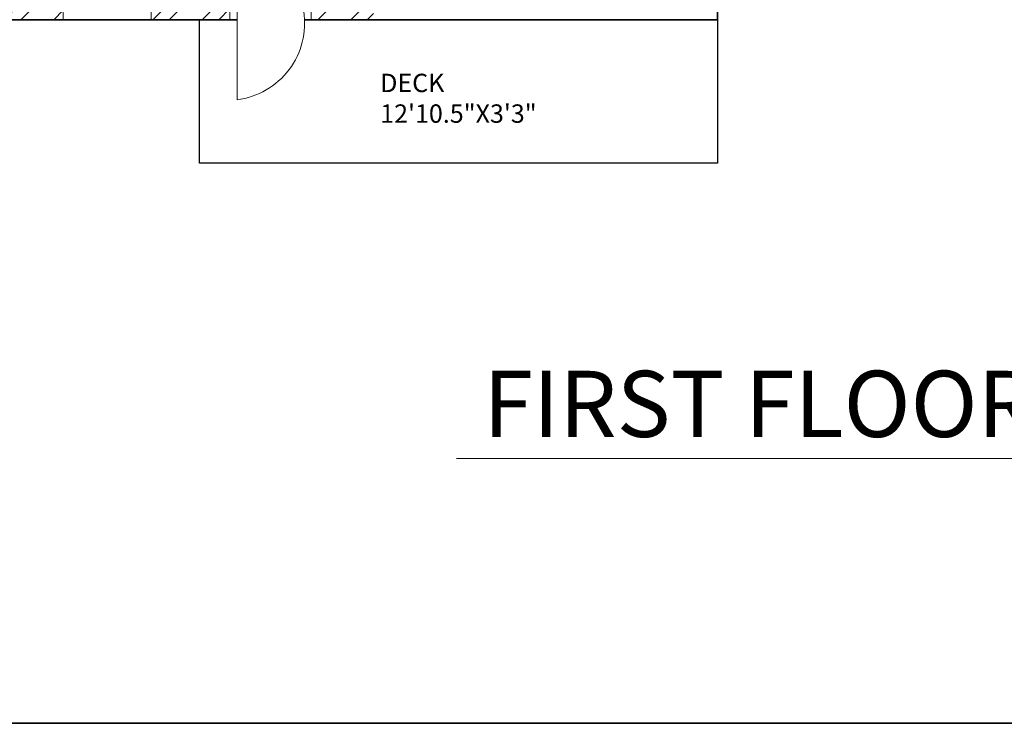
# Model space of a CAD drawing. Units: inches. Extents: x 2120 to 4013, y 1390 to 3019.
# Tile 9 of 59: x 2448 to 2716, y 1390 to 1582. Entities that reach past the tile are written whole.
import ezdxf

# ---------------------------------------------------------------- set-up
doc = ezdxf.new("R2010")
doc.units = ezdxf.units.IN
for name, color, linetype, lineweight in [('A-ANNO-TEXT', 7, 'Continuous', 18), ('A-ANNO-TTLB', 7, 'Continuous', 35), ('A-AREA-IDEN', 7, 'Continuous', 18), ('A-DOOR', 3, 'Continuous', 18), ('A-FLOR-DECK', 7, 'Continuous', 25), ('A-GLAZ', 4, 'Continuous', 18), ('A-WALL', 7, 'Continuous', 35), ('A-WALL-PATT', 252, 'Continuous', 13)]:
    doc.layers.add(name, color=color, linetype=linetype, lineweight=lineweight)
doc.styles.get("Standard").update_dxf_attribs({"font": 'arial.ttf'})

# ---------------------------------------------------------------- blocks, each defined once
blk = doc.blocks.new('DOOR-SWING-24IN-91p57DEG')
for p, q in [((0, 26.25), (0, 21.75)), ((22.12, 21.75), (22.12, 26.25)), ((22.12, 26.25), (22.12, 24)), ((0, 21.75), (0, 24)), ((0, 24), (2, 24)), ((2, 24), (2, 0)), ((22.12, 24), (20.12, 24))]:
    blk.add_line(p, q)
blk.add_arc((-0.62, 20.81), 20.98, 277.1643, 8.7385)
blk = doc.blocks.new('WIN-PLAN-24IN-03')
for p, q in [((9, 24), (0, 24)), ((0, 24), (4.5, 24)), ((4.5, 24), (4.5, 0)), ((9, 0), (0, 0)), ((4.5, 0), (9, 0))]:
    blk.add_line(p, q)

msp = doc.modelspace()

# ---------------------------------------------------------------- hatches: boundary and pattern name
at = {"layer": 'A-WALL-PATT'}
h = msp.add_hatch(dxfattribs=at)
h.set_pattern_fill('ANSI32', color=256)
h.paths.add_polyline_path([(2271.7331, 2343.531), (2283.3788, 2343.531), (2283.3788, 2348.031), (2283.3788, 2352.5306), (2262.7331, 2352.5306), (2262.7331, 2182.638), (2267.2331, 2182.638), (2271.7331, 2182.638), (2271.7331, 2219.031), (2391.7331, 2219.031), (2391.7331, 2214.189), (2393.9831, 2214.189), (2396.2331, 2214.189), (2396.2331, 2219.031), (2420.2331, 2219.031), (2420.2331, 2225.7535), (2417.2197, 2225.7535), (2415.7331, 2225.7535), (2415.7331, 2223.5306), (2271.7331, 2223.5306)])
h.paths.add_polyline_path([(2380.0942, 2352.5306), (2343.3788, 2352.5306), (2343.3788, 2343.531), (2363.2331, 2343.531), (2363.2331, 2288.8489), (2365.4831, 2288.8489), (2367.7331, 2288.8489), (2367.7331, 2343.531), (2380.0942, 2343.531)], flags=17)
h.paths.add_polyline_path([(2432.4339, 2352.5306), (2404.0943, 2352.5306), (2404.0943, 2343.531), (2415.7331, 2343.531), (2415.7331, 2264.0306), (2367.7331, 2264.0306), (2367.7331, 2266.4872), (2363.2331, 2266.4872), (2363.2331, 2259.531), (2367.7331, 2259.531), (2415.7331, 2259.531), (2415.7331, 2255.0658), (2420.2331, 2255.0658), (2420.2331, 2259.531), (2424.5717, 2259.531), (2424.5717, 2261.781), (2424.5717, 2264.0306), (2420.2331, 2264.0306), (2420.2331, 2343.531), (2432.4339, 2343.531)])
h.paths.add_polyline_path([(2508.9115, 2352.5306), (2456.4339, 2352.5306), (2456.4339, 2343.531), (2468.2331, 2343.531), (2468.2331, 2264.0306), (2448.0487, 2264.0306), (2448.0487, 2259.531), (2468.2331, 2259.531), (2468.2331, 2255.5496), (2472.7331, 2255.5496), (2472.7331, 2343.531), (2508.9115, 2343.531)])
h.paths.add_polyline_path([(2637.7331, 2352.5306), (2544.9116, 2352.5306), (2544.9116, 2343.531), (2589.7331, 2343.531), (2633.2331, 2343.531), (2637.7331, 2343.531)])
h.paths.add_polyline_path([(2594.2331, 2343.5306), (2589.7331, 2343.5306), (2589.7331, 2259.5306), (2589.7331, 2252.4915), (2591.9831, 2252.4915), (2594.2331, 2252.4915)])
h.paths.add_polyline_path([(2637.7331, 2223.5306), (2594.2331, 2223.5306), (2594.2331, 2230.1988), (2591.9831, 2230.1988), (2589.7331, 2230.1988), (2589.7331, 2223.5306), (2472.7331, 2223.5306), (2468.2331, 2223.5306), (2468.2331, 2219.031), (2628.7331, 2219.031), (2628.7331, 2138.031), (2637.7331, 2138.031)])
h.paths.add_polyline_path([(3822.6535, 2458.4402), (3874.9468, 2458.4402), (3874.9468, 2476.9866), (3822.6535, 2476.9866)], flags=9)
h.paths.add_polyline_path([(3834.6921, 2781.8174), (3935.9206, 2781.8174), (3935.9206, 2800.3638), (3834.6921, 2800.3638)], flags=9)
h.paths.add_polyline_path([(3832.2843, 2837.9683), (3884.5776, 2837.9683), (3884.5776, 2856.5146), (3832.2843, 2856.5146)], flags=9)
h.paths.add_polyline_path([(3830.9388, 2861.4782), (3956.8958, 2861.4782), (3956.8958, 2880.0245), (3830.9388, 2880.0245)], flags=9)
h.paths.add_polyline_path([(3870.6966, 2352.5752), (3887.9272, 2352.5752), (3887.9272, 2377.3037), (3870.6966, 2377.3037)], flags=9)
h.paths.add_polyline_path([(3289.2701, 2413.161), (3435.2223, 2413.161), (3435.2223, 2450.2538), (3289.2701, 2450.2538)], flags=9)
h.paths.add_polyline_path([(2487.6944, 2414.3601), (2637.8335, 2414.3601), (2637.8335, 2451.4528), (2487.6944, 2451.4528)], flags=9)
h.paths.add_polyline_path([(2567.3724, 1457.9199), (2815.296, 1457.9199), (2815.296, 1495.0127), (2567.3724, 1495.0127)], flags=9)
h.paths.add_polyline_path([(2655.3825, 2093.2363), (2685.9555, 2093.2363), (2685.9555, 2111.8937), (2655.3825, 2111.8937)], flags=9)
h.paths.add_polyline_path([(2543.9218, 1550.6671), (2587.8406, 1550.6671), (2587.8406, 1569.3244), (2543.9218, 1569.3244)], flags=9)
h.paths.add_polyline_path([(2905.1384, 1543.8113), (2949.0572, 1543.8113), (2949.0572, 1562.4686), (2905.1384, 1562.4686)], flags=9)
h.paths.add_polyline_path([(2736.4118, 1702.4736), (2784.2153, 1702.4736), (2784.2153, 1721.1309), (2736.4118, 1721.1309)], flags=9)
h.paths.add_polyline_path([(2912.8666, 1710.4168), (2951.707, 1710.4168), (2951.707, 1729.0741), (2912.8666, 1729.0741)], flags=9)
h.paths.add_polyline_path([(2923.5785, 1763.5038), (2959.7279, 1763.5038), (2959.7279, 1782.1611), (2923.5785, 1782.1611)], flags=9)
h.paths.add_polyline_path([(2925.2114, 1809.6137), (2967.1861, 1809.6137), (2967.1861, 1828.271), (2925.2114, 1828.271)], flags=9)
h.paths.add_polyline_path([(2996.2711, 1878.9003), (2996.2711, 1913.109), (2977.6138, 1913.109), (2977.6138, 1878.9003)], flags=9)
h.paths.add_polyline_path([(2883.0859, 1895.7192), (2927.1855, 1895.7192), (2927.1855, 1914.3766), (2883.0859, 1914.3766)], flags=9)
h.paths.add_polyline_path([(2787.3924, 1810.8013), (2841.0213, 1810.8013), (2841.0213, 1829.4587), (2787.3924, 1829.4587)], flags=9)
h.paths.add_polyline_path([(2775.6399, 2101.7395), (2829.2689, 2101.7395), (2829.2689, 2120.3968), (2775.6399, 2120.3968)], flags=9)
h.paths.add_polyline_path([(2913.0263, 2075.817), (2951.8667, 2075.817), (2951.8667, 2094.4744), (2913.0263, 2094.4744)], flags=9)
h.paths.add_polyline_path([(2929.966, 2133.3669), (2966.1154, 2133.3669), (2966.1154, 2152.0243), (2929.966, 2152.0243)], flags=9)
h.paths.add_polyline_path([(2932.7502, 2182.6088), (2968.8996, 2182.6088), (2968.8996, 2201.2662), (2932.7502, 2201.2662)], flags=9)
h.paths.add_polyline_path([(2996.0681, 2266.3173), (2996.0681, 2300.5261), (2977.4108, 2300.5261), (2977.4108, 2266.3173)], flags=9)
h.paths.add_polyline_path([(2885.1039, 2279.2186), (2929.2035, 2279.2186), (2929.2035, 2297.8759), (2885.1039, 2297.8759)], flags=9)
h.paths.add_polyline_path([(2735.7042, 2218.3197), (2783.5078, 2218.3197), (2783.5078, 2236.9771), (2735.7042, 2236.9771)], flags=9)
h.paths.add_polyline_path([(2635.6049, 2044.0085), (2648.9678, 2044.0085), (2648.9678, 2054.312), (2635.6049, 2054.312)], flags=9)
h.paths.add_polyline_path([(2714.0148, 1923.0473), (2727.3777, 1923.0473), (2727.3777, 1933.3508), (2714.0148, 1933.3508)], flags=9)
h.paths.add_polyline_path([(2709.0345, 1988.1628), (2722.3974, 1988.1628), (2722.3974, 1998.4663), (2709.0345, 1998.4663)], flags=9)
h.paths.add_polyline_path([(2592.8935, 1962.1763), (2606.2564, 1962.1763), (2606.2564, 1972.4799), (2592.8935, 1972.4799)], flags=9)
h.paths.add_polyline_path([(2618.3996, 1985.9724), (2644.1942, 1985.9724), (2644.1942, 1996.2759), (2618.3996, 1996.2759)], flags=9)
h.paths.add_polyline_path([(2601.279, 1920.5869), (2614.6419, 1920.5869), (2614.6419, 1930.8904), (2601.279, 1930.8904)], flags=9)
h.paths.add_polyline_path([(2692.3278, 1932.7645), (2704.5311, 1932.7645), (2704.5311, 1943.0681), (2692.3278, 1943.0681)], flags=9)
h.paths.add_polyline_path([(2311.122, 1672.7318), (2355.0408, 1672.7318), (2355.0408, 1691.3892), (2311.122, 1691.3892)], flags=9)
h.paths.add_polyline_path([(2456.2551, 1632.3198), (2492.4796, 1632.3198), (2492.4796, 1650.9772), (2456.2551, 1650.9772)], flags=9)
h.paths.add_polyline_path([(2401.0766, 1631.4793), (2437.301, 1631.4793), (2437.301, 1650.1367), (2401.0766, 1650.1367)], flags=9)
h.paths.add_polyline_path([(2546.7054, 1700.9235), (2594.509, 1700.9235), (2594.509, 1719.5809), (2546.7054, 1719.5809)], flags=9)
h.paths.add_polyline_path([(2445.4866, 1766.9937), (2497.5261, 1766.9937), (2497.5261, 1785.651), (2445.4866, 1785.651)], flags=9)
h.paths.add_polyline_path([(2287.9992, 1739.7675), (2326.8396, 1739.7675), (2326.8396, 1758.4248), (2287.9992, 1758.4248)], flags=9)
h.paths.add_polyline_path([(2458.5279, 1924.7607), (2510.5675, 1924.7607), (2510.5675, 1943.4181), (2458.5279, 1943.4181)], flags=9)
h.paths.add_polyline_path([(2309.2811, 1902.7642), (2345.4305, 1902.7642), (2345.4305, 1921.4215), (2309.2811, 1921.4215)], flags=9)
h.paths.add_polyline_path([(2490.7554, 2018.9392), (2530.7896, 2018.9392), (2530.7896, 2037.5965), (2490.7554, 2037.5965)], flags=9)
h.paths.add_polyline_path([(2402.143, 2024.7393), (2438.5414, 2024.7393), (2438.5414, 2043.3966), (2402.143, 2043.3966)], flags=9)
h.paths.add_polyline_path([(2287.856, 1931.7926), (2326.6964, 1931.7926), (2326.6964, 1950.4499), (2287.856, 1950.4499)], flags=9)
h.paths.add_polyline_path([(2281.7979, 2193.5771), (2320.6383, 2193.5771), (2320.6383, 2212.2344), (2281.7979, 2212.2344)], flags=25)
h.paths.add_polyline_path([(2484.0754, 2093.892), (2536.115, 2093.892), (2536.115, 2112.5494), (2484.0754, 2112.5494)], flags=9)
h.paths.add_polyline_path([(2624.7948, 2281.8639), (2624.7948, 2311.4137), (2606.1375, 2311.4137), (2606.1375, 2281.8639)], flags=9)
h.paths.add_polyline_path([(2507.5036, 2290.3639), (2541.934, 2290.3639), (2541.934, 2309.0212), (2507.5036, 2309.0212)], flags=9)
h.paths.add_polyline_path([(2423.1076, 2285.2202), (2459.332, 2285.2202), (2459.332, 2303.8776), (2423.1076, 2303.8776)], flags=9)
h.paths.add_polyline_path([(2374.5467, 2289.6272), (2410.7711, 2289.6272), (2410.7711, 2308.2846), (2374.5467, 2308.2846)], flags=25)
h.paths.add_polyline_path([(2277.4907, 2227.5651), (2316.3311, 2227.5651), (2316.3311, 2246.2224), (2277.4907, 2246.2224)], flags=25)
h.paths.add_polyline_path([(2655.3825, 2093.2367), (2685.9555, 2093.2367), (2685.9555, 2111.894), (2655.3825, 2111.894)], flags=9)
h.paths.add_polyline_path([(2543.9217, 1550.6674), (2587.8406, 1550.6674), (2587.8406, 1569.3247), (2543.9217, 1569.3247)], flags=9)
h.paths.add_polyline_path([(2905.1384, 1543.8116), (2949.0572, 1543.8116), (2949.0572, 1562.4689), (2905.1384, 1562.4689)], flags=9)
h.paths.add_polyline_path([(2736.4118, 1702.4739), (2784.2153, 1702.4739), (2784.2153, 1721.1312), (2736.4118, 1721.1312)], flags=9)
h.paths.add_polyline_path([(2912.8666, 1710.4171), (2951.707, 1710.4171), (2951.707, 1729.0744), (2912.8666, 1729.0744)], flags=9)
h.paths.add_polyline_path([(2923.5785, 1763.5041), (2959.7279, 1763.5041), (2959.7279, 1782.1614), (2923.5785, 1782.1614)], flags=9)
h.paths.add_polyline_path([(2925.2114, 1809.614), (2967.1861, 1809.614), (2967.1861, 1828.2713), (2925.2114, 1828.2713)], flags=9)
h.paths.add_polyline_path([(2996.2711, 1878.9006), (2996.2711, 1913.1094), (2977.6137, 1913.1094), (2977.6137, 1878.9006)], flags=9)
h.paths.add_polyline_path([(2883.0859, 1895.7195), (2927.1855, 1895.7195), (2927.1855, 1914.3769), (2883.0859, 1914.3769)], flags=9)
h.paths.add_polyline_path([(2787.3924, 1810.8016), (2841.0213, 1810.8016), (2841.0213, 1829.459), (2787.3924, 1829.459)], flags=9)
h.paths.add_polyline_path([(2775.6399, 2101.7398), (2829.2688, 2101.7398), (2829.2688, 2120.3971), (2775.6399, 2120.3971)], flags=9)
h.paths.add_polyline_path([(2913.0263, 2075.8173), (2951.8667, 2075.8173), (2951.8667, 2094.4747), (2913.0263, 2094.4747)], flags=9)
h.paths.add_polyline_path([(2929.966, 2133.3672), (2966.1154, 2133.3672), (2966.1154, 2152.0246), (2929.966, 2152.0246)], flags=9)
h.paths.add_polyline_path([(2932.7502, 2182.6091), (2968.8996, 2182.6091), (2968.8996, 2201.2665), (2932.7502, 2201.2665)], flags=9)
h.paths.add_polyline_path([(2996.0681, 2266.3176), (2996.0681, 2300.5264), (2977.4108, 2300.5264), (2977.4108, 2266.3176)], flags=9)
h.paths.add_polyline_path([(2885.1039, 2279.2189), (2929.2035, 2279.2189), (2929.2035, 2297.8762), (2885.1039, 2297.8762)], flags=9)
h.paths.add_polyline_path([(2735.7042, 2218.32), (2783.5078, 2218.32), (2783.5078, 2236.9774), (2735.7042, 2236.9774)], flags=9)
h.paths.add_polyline_path([(2635.6048, 2044.0088), (2648.9677, 2044.0088), (2648.9677, 2054.3123), (2635.6048, 2054.3123)], flags=9)
h.paths.add_polyline_path([(2714.0148, 1923.0476), (2727.3777, 1923.0476), (2727.3777, 1933.3511), (2714.0148, 1933.3511)], flags=9)
h.paths.add_polyline_path([(2709.0345, 1988.1631), (2722.3974, 1988.1631), (2722.3974, 1998.4666), (2709.0345, 1998.4666)], flags=9)
h.paths.add_polyline_path([(2592.8935, 1962.1766), (2606.2564, 1962.1766), (2606.2564, 1972.4802), (2592.8935, 1972.4802)], flags=9)
h.paths.add_polyline_path([(2618.3995, 1985.9727), (2644.1942, 1985.9727), (2644.1942, 1996.2762), (2618.3995, 1996.2762)], flags=9)
h.paths.add_polyline_path([(2601.279, 1920.5872), (2614.6419, 1920.5872), (2614.6419, 1930.8908), (2601.279, 1930.8908)], flags=9)
h.paths.add_polyline_path([(2692.3278, 1932.7648), (2704.5311, 1932.7648), (2704.5311, 1943.0684), (2692.3278, 1943.0684)], flags=9)
h.paths.add_polyline_path([(2311.122, 1672.7321), (2355.0408, 1672.7321), (2355.0408, 1691.3895), (2311.122, 1691.3895)], flags=9)
h.paths.add_polyline_path([(2456.2551, 1632.3201), (2492.4795, 1632.3201), (2492.4795, 1650.9775), (2456.2551, 1650.9775)], flags=9)
h.paths.add_polyline_path([(2401.0766, 1631.4796), (2437.301, 1631.4796), (2437.301, 1650.137), (2401.0766, 1650.137)], flags=9)
h.paths.add_polyline_path([(2546.7054, 1700.9238), (2594.509, 1700.9238), (2594.509, 1719.5812), (2546.7054, 1719.5812)], flags=9)
h.paths.add_polyline_path([(2445.4866, 1766.994), (2497.5261, 1766.994), (2497.5261, 1785.6513), (2445.4866, 1785.6513)], flags=9)
h.paths.add_polyline_path([(2287.9992, 1739.7678), (2326.8396, 1739.7678), (2326.8396, 1758.4251), (2287.9992, 1758.4251)], flags=9)
h.paths.add_polyline_path([(2458.5279, 1924.7611), (2510.5675, 1924.7611), (2510.5675, 1943.4184), (2458.5279, 1943.4184)], flags=9)
h.paths.add_polyline_path([(2309.2811, 1902.7645), (2345.4305, 1902.7645), (2345.4305, 1921.4218), (2309.2811, 1921.4218)], flags=9)
h.paths.add_polyline_path([(2490.7554, 2018.9395), (2530.7895, 2018.9395), (2530.7895, 2037.5968), (2490.7554, 2037.5968)], flags=9)
h.paths.add_polyline_path([(2402.143, 2024.7396), (2438.5413, 2024.7396), (2438.5413, 2043.3969), (2402.143, 2043.3969)], flags=9)
h.paths.add_polyline_path([(2287.856, 1931.7929), (2326.6964, 1931.7929), (2326.6964, 1950.4502), (2287.856, 1950.4502)], flags=9)
h.paths.add_polyline_path([(2281.7979, 2193.5774), (2320.6383, 2193.5774), (2320.6383, 2212.2347), (2281.7979, 2212.2347)], flags=25)
h.paths.add_polyline_path([(2484.0754, 2093.8924), (2536.115, 2093.8924), (2536.115, 2112.5497), (2484.0754, 2112.5497)], flags=9)
h.paths.add_polyline_path([(2624.7948, 2281.8642), (2624.7948, 2311.414), (2606.1374, 2311.414), (2606.1374, 2281.8642)], flags=9)
h.paths.add_polyline_path([(2507.5035, 2290.3642), (2541.934, 2290.3642), (2541.934, 2309.0215), (2507.5035, 2309.0215)], flags=9)
h.paths.add_polyline_path([(2423.1075, 2285.2205), (2459.332, 2285.2205), (2459.332, 2303.8779), (2423.1075, 2303.8779)], flags=9)
h.paths.add_polyline_path([(2374.5467, 2289.6275), (2410.7711, 2289.6275), (2410.7711, 2308.2849), (2374.5467, 2308.2849)], flags=25)
h.paths.add_polyline_path([(2277.4907, 2227.5654), (2316.3311, 2227.5654), (2316.3311, 2246.2227), (2277.4907, 2246.2227)], flags=25)
h = msp.add_hatch(dxfattribs=at)
h.set_pattern_fill('ANSI32', color=256)
h.paths.add_polyline_path([(2271.7331, 1980.389), (2262.7331, 1980.389), (2262.7331, 1912.8434), (2267.2331, 1912.8434), (2271.7331, 1912.8434), (2271.7331, 1922.531), (2351.2331, 1922.531), (2351.2331, 1901.4728), (2355.7331, 1901.4728), (2355.7331, 1922.531), (2357.9815, 1922.531), (2357.9815, 1926.5306), (2271.7331, 1926.5306)])
h.paths.add_polyline_path([(2589.2331, 1949.1622), (2584.7331, 1949.1622), (2580.2331, 1949.1622), (2580.2331, 1874.5306), (2355.7331, 1874.5306), (2355.7331, 1880.1922), (2351.2331, 1880.1922), (2351.2331, 1874.5306), (2271.7331, 1874.5306), (2271.7331, 1888.8431), (2262.7331, 1888.8431), (2262.7331, 1842.2909), (2267.2331, 1842.2909), (2271.7331, 1842.2909), (2271.7331, 1865.531), (2415.7331, 1865.531), (2415.7331, 1779.7286), (2420.2331, 1779.7286), (2420.2331, 1865.531), (2589.2331, 1865.531)])
h.paths.add_polyline_path([(2271.7331, 1782.2906), (2262.7331, 1782.2906), (2262.7331, 1711.4639), (2267.2331, 1711.4639), (2271.7331, 1711.4639), (2271.7331, 1738.031), (2420.2331, 1738.031), (2420.2331, 1742.531), (2420.2331, 1747.3376), (2417.9831, 1747.3376), (2415.7331, 1747.3376), (2415.7331, 1742.5306), (2271.7331, 1742.5306)])
h.paths.add_polyline_path([(2271.7331, 1627.031), (2362.3957, 1627.031), (2362.3957, 1629.281), (2362.3957, 1631.5306), (2271.7331, 1631.5306), (2271.7331, 1675.4636), (2262.7331, 1675.4636), (2262.7331, 1581.531), (2405.3032, 1581.531), (2405.3032, 1586.031), (2405.3032, 1590.5306), (2396.2331, 1590.5306), (2396.2331, 1691.4513), (2418.7206, 1691.4513), (2418.7206, 1695.951), (2396.2331, 1695.951), (2391.7331, 1695.951), (2391.7331, 1631.5306), (2386.7425, 1631.5306), (2386.7425, 1629.2806), (2386.7425, 1627.031), (2391.7331, 1627.031), (2391.7331, 1586.1709), (2271.7331, 1586.1709)])
h.paths.add_polyline_path([(2459.6703, 1590.5306), (2429.3032, 1590.5306), (2429.3032, 1581.531), (2459.6703, 1581.531), (2459.6703, 1586.031)])
h.paths.add_polyline_path([(2501.2331, 1590.531), (2501.2331, 1665.0195), (2498.9831, 1665.0195), (2496.7331, 1665.0195), (2496.7331, 1590.5306), (2483.8201, 1590.5306), (2483.8201, 1590.1579), (2483.6704, 1590.1579), (2483.6704, 1581.531), (2505.0196, 1581.531), (2505.0196, 1583.781), (2505.0196, 1586.0306), (2501.2331, 1586.0306)])
h.paths.add_polyline_path([(2544.1361, 1583.781), (2544.1361, 1586.0306), (2527.1368, 1586.0306), (2527.1368, 1583.7806), (2527.1368, 1581.531), (2544.1361, 1581.531)])
h.paths.add_polyline_path([(3822.6535, 2458.4402), (3874.9468, 2458.4402), (3874.9468, 2476.9866), (3822.6535, 2476.9866)], flags=9)
h.paths.add_polyline_path([(3834.6921, 2781.8174), (3935.9206, 2781.8174), (3935.9206, 2800.3638), (3834.6921, 2800.3638)], flags=9)
h.paths.add_polyline_path([(3832.2843, 2837.9683), (3884.5776, 2837.9683), (3884.5776, 2856.5146), (3832.2843, 2856.5146)], flags=9)
h.paths.add_polyline_path([(3830.9388, 2861.4782), (3956.8958, 2861.4782), (3956.8958, 2880.0245), (3830.9388, 2880.0245)], flags=9)
h.paths.add_polyline_path([(3870.6966, 2352.5752), (3887.9272, 2352.5752), (3887.9272, 2377.3037), (3870.6966, 2377.3037)], flags=9)
h.paths.add_polyline_path([(3289.2701, 2413.161), (3435.2223, 2413.161), (3435.2223, 2450.2538), (3289.2701, 2450.2538)], flags=9)
h.paths.add_polyline_path([(2487.6944, 2414.3601), (2637.8335, 2414.3601), (2637.8335, 2451.4528), (2487.6944, 2451.4528)], flags=9)
h.paths.add_polyline_path([(2567.3724, 1457.9199), (2815.296, 1457.9199), (2815.296, 1495.0127), (2567.3724, 1495.0127)], flags=9)
h.paths.add_polyline_path([(2655.3825, 2093.2363), (2685.9555, 2093.2363), (2685.9555, 2111.8937), (2655.3825, 2111.8937)], flags=9)
h.paths.add_polyline_path([(2543.9218, 1550.6671), (2587.8406, 1550.6671), (2587.8406, 1569.3244), (2543.9218, 1569.3244)], flags=9)
h.paths.add_polyline_path([(2905.1384, 1543.8113), (2949.0572, 1543.8113), (2949.0572, 1562.4686), (2905.1384, 1562.4686)], flags=9)
h.paths.add_polyline_path([(2736.4118, 1702.4736), (2784.2153, 1702.4736), (2784.2153, 1721.1309), (2736.4118, 1721.1309)], flags=9)
h.paths.add_polyline_path([(2912.8666, 1710.4168), (2951.707, 1710.4168), (2951.707, 1729.0741), (2912.8666, 1729.0741)], flags=9)
h.paths.add_polyline_path([(2923.5785, 1763.5038), (2959.7279, 1763.5038), (2959.7279, 1782.1611), (2923.5785, 1782.1611)], flags=9)
h.paths.add_polyline_path([(2925.2114, 1809.6137), (2967.1861, 1809.6137), (2967.1861, 1828.271), (2925.2114, 1828.271)], flags=9)
h.paths.add_polyline_path([(2996.2711, 1878.9003), (2996.2711, 1913.109), (2977.6138, 1913.109), (2977.6138, 1878.9003)], flags=9)
h.paths.add_polyline_path([(2883.0859, 1895.7192), (2927.1855, 1895.7192), (2927.1855, 1914.3766), (2883.0859, 1914.3766)], flags=9)
h.paths.add_polyline_path([(2787.3924, 1810.8013), (2841.0213, 1810.8013), (2841.0213, 1829.4587), (2787.3924, 1829.4587)], flags=9)
h.paths.add_polyline_path([(2775.6399, 2101.7395), (2829.2689, 2101.7395), (2829.2689, 2120.3968), (2775.6399, 2120.3968)], flags=9)
h.paths.add_polyline_path([(2913.0263, 2075.817), (2951.8667, 2075.817), (2951.8667, 2094.4744), (2913.0263, 2094.4744)], flags=9)
h.paths.add_polyline_path([(2929.966, 2133.3669), (2966.1154, 2133.3669), (2966.1154, 2152.0243), (2929.966, 2152.0243)], flags=9)
h.paths.add_polyline_path([(2932.7502, 2182.6088), (2968.8996, 2182.6088), (2968.8996, 2201.2662), (2932.7502, 2201.2662)], flags=9)
h.paths.add_polyline_path([(2996.0681, 2266.3173), (2996.0681, 2300.5261), (2977.4108, 2300.5261), (2977.4108, 2266.3173)], flags=9)
h.paths.add_polyline_path([(2885.1039, 2279.2186), (2929.2035, 2279.2186), (2929.2035, 2297.8759), (2885.1039, 2297.8759)], flags=9)
h.paths.add_polyline_path([(2735.7042, 2218.3197), (2783.5078, 2218.3197), (2783.5078, 2236.9771), (2735.7042, 2236.9771)], flags=9)
h.paths.add_polyline_path([(2635.6049, 2044.0085), (2648.9678, 2044.0085), (2648.9678, 2054.312), (2635.6049, 2054.312)], flags=9)
h.paths.add_polyline_path([(2714.0148, 1923.0473), (2727.3777, 1923.0473), (2727.3777, 1933.3508), (2714.0148, 1933.3508)], flags=9)
h.paths.add_polyline_path([(2709.0345, 1988.1628), (2722.3974, 1988.1628), (2722.3974, 1998.4663), (2709.0345, 1998.4663)], flags=9)
h.paths.add_polyline_path([(2592.8935, 1962.1763), (2606.2564, 1962.1763), (2606.2564, 1972.4799), (2592.8935, 1972.4799)], flags=9)
h.paths.add_polyline_path([(2618.3996, 1985.9724), (2644.1942, 1985.9724), (2644.1942, 1996.2759), (2618.3996, 1996.2759)], flags=9)
h.paths.add_polyline_path([(2601.279, 1920.5869), (2614.6419, 1920.5869), (2614.6419, 1930.8904), (2601.279, 1930.8904)], flags=9)
h.paths.add_polyline_path([(2692.3278, 1932.7645), (2704.5311, 1932.7645), (2704.5311, 1943.0681), (2692.3278, 1943.0681)], flags=9)
h.paths.add_polyline_path([(2311.122, 1672.7318), (2355.0408, 1672.7318), (2355.0408, 1691.3892), (2311.122, 1691.3892)], flags=25)
h.paths.add_polyline_path([(2456.2551, 1632.3198), (2492.4796, 1632.3198), (2492.4796, 1650.9772), (2456.2551, 1650.9772)], flags=9)
h.paths.add_polyline_path([(2401.0766, 1631.4793), (2437.301, 1631.4793), (2437.301, 1650.1367), (2401.0766, 1650.1367)], flags=9)
h.paths.add_polyline_path([(2546.7054, 1700.9235), (2594.509, 1700.9235), (2594.509, 1719.5809), (2546.7054, 1719.5809)], flags=9)
h.paths.add_polyline_path([(2445.4866, 1766.9937), (2497.5261, 1766.9937), (2497.5261, 1785.651), (2445.4866, 1785.651)], flags=9)
h.paths.add_polyline_path([(2287.9992, 1739.7675), (2326.8396, 1739.7675), (2326.8396, 1758.4248), (2287.9992, 1758.4248)], flags=24)
h.paths.add_polyline_path([(2458.5279, 1924.7607), (2510.5675, 1924.7607), (2510.5675, 1943.4181), (2458.5279, 1943.4181)], flags=25)
h.paths.add_polyline_path([(2309.2811, 1902.7642), (2345.4305, 1902.7642), (2345.4305, 1921.4215), (2309.2811, 1921.4215)], flags=25)
h.paths.add_polyline_path([(2490.7554, 2018.9392), (2530.7896, 2018.9392), (2530.7896, 2037.5965), (2490.7554, 2037.5965)], flags=9)
h.paths.add_polyline_path([(2402.143, 2024.7393), (2438.5414, 2024.7393), (2438.5414, 2043.3966), (2402.143, 2043.3966)], flags=9)
h.paths.add_polyline_path([(2287.856, 1931.7926), (2326.6964, 1931.7926), (2326.6964, 1950.4499), (2287.856, 1950.4499)], flags=25)
h.paths.add_polyline_path([(2281.7979, 2193.5771), (2320.6383, 2193.5771), (2320.6383, 2212.2344), (2281.7979, 2212.2344)], flags=9)
h.paths.add_polyline_path([(2484.0754, 2093.892), (2536.115, 2093.892), (2536.115, 2112.5494), (2484.0754, 2112.5494)], flags=9)
h.paths.add_polyline_path([(2624.7948, 2281.8639), (2624.7948, 2311.4137), (2606.1375, 2311.4137), (2606.1375, 2281.8639)], flags=9)
h.paths.add_polyline_path([(2507.5036, 2290.3639), (2541.934, 2290.3639), (2541.934, 2309.0212), (2507.5036, 2309.0212)], flags=9)
h.paths.add_polyline_path([(2423.1076, 2285.2202), (2459.332, 2285.2202), (2459.332, 2303.8776), (2423.1076, 2303.8776)], flags=9)
h.paths.add_polyline_path([(2374.5467, 2289.6272), (2410.7711, 2289.6272), (2410.7711, 2308.2846), (2374.5467, 2308.2846)], flags=9)
h.paths.add_polyline_path([(2277.4907, 2227.5651), (2316.3311, 2227.5651), (2316.3311, 2246.2224), (2277.4907, 2246.2224)], flags=9)
h.paths.add_polyline_path([(2655.3825, 2093.2367), (2685.9555, 2093.2367), (2685.9555, 2111.894), (2655.3825, 2111.894)], flags=9)
h.paths.add_polyline_path([(2543.9217, 1550.6674), (2587.8406, 1550.6674), (2587.8406, 1569.3247), (2543.9217, 1569.3247)], flags=9)
h.paths.add_polyline_path([(2905.1384, 1543.8116), (2949.0572, 1543.8116), (2949.0572, 1562.4689), (2905.1384, 1562.4689)], flags=9)
h.paths.add_polyline_path([(2736.4118, 1702.4739), (2784.2153, 1702.4739), (2784.2153, 1721.1312), (2736.4118, 1721.1312)], flags=9)
h.paths.add_polyline_path([(2912.8666, 1710.4171), (2951.707, 1710.4171), (2951.707, 1729.0744), (2912.8666, 1729.0744)], flags=9)
h.paths.add_polyline_path([(2923.5785, 1763.5041), (2959.7279, 1763.5041), (2959.7279, 1782.1614), (2923.5785, 1782.1614)], flags=9)
h.paths.add_polyline_path([(2925.2114, 1809.614), (2967.1861, 1809.614), (2967.1861, 1828.2713), (2925.2114, 1828.2713)], flags=9)
h.paths.add_polyline_path([(2996.2711, 1878.9006), (2996.2711, 1913.1094), (2977.6137, 1913.1094), (2977.6137, 1878.9006)], flags=9)
h.paths.add_polyline_path([(2883.0859, 1895.7195), (2927.1855, 1895.7195), (2927.1855, 1914.3769), (2883.0859, 1914.3769)], flags=9)
h.paths.add_polyline_path([(2787.3924, 1810.8016), (2841.0213, 1810.8016), (2841.0213, 1829.459), (2787.3924, 1829.459)], flags=9)
h.paths.add_polyline_path([(2775.6399, 2101.7398), (2829.2688, 2101.7398), (2829.2688, 2120.3971), (2775.6399, 2120.3971)], flags=9)
h.paths.add_polyline_path([(2913.0263, 2075.8173), (2951.8667, 2075.8173), (2951.8667, 2094.4747), (2913.0263, 2094.4747)], flags=9)
h.paths.add_polyline_path([(2929.966, 2133.3672), (2966.1154, 2133.3672), (2966.1154, 2152.0246), (2929.966, 2152.0246)], flags=9)
h.paths.add_polyline_path([(2932.7502, 2182.6091), (2968.8996, 2182.6091), (2968.8996, 2201.2665), (2932.7502, 2201.2665)], flags=9)
h.paths.add_polyline_path([(2996.0681, 2266.3176), (2996.0681, 2300.5264), (2977.4108, 2300.5264), (2977.4108, 2266.3176)], flags=9)
h.paths.add_polyline_path([(2885.1039, 2279.2189), (2929.2035, 2279.2189), (2929.2035, 2297.8762), (2885.1039, 2297.8762)], flags=9)
h.paths.add_polyline_path([(2735.7042, 2218.32), (2783.5078, 2218.32), (2783.5078, 2236.9774), (2735.7042, 2236.9774)], flags=9)
h.paths.add_polyline_path([(2635.6048, 2044.0088), (2648.9677, 2044.0088), (2648.9677, 2054.3123), (2635.6048, 2054.3123)], flags=9)
h.paths.add_polyline_path([(2714.0148, 1923.0476), (2727.3777, 1923.0476), (2727.3777, 1933.3511), (2714.0148, 1933.3511)], flags=9)
h.paths.add_polyline_path([(2709.0345, 1988.1631), (2722.3974, 1988.1631), (2722.3974, 1998.4666), (2709.0345, 1998.4666)], flags=9)
h.paths.add_polyline_path([(2592.8935, 1962.1766), (2606.2564, 1962.1766), (2606.2564, 1972.4802), (2592.8935, 1972.4802)], flags=9)
h.paths.add_polyline_path([(2618.3995, 1985.9727), (2644.1942, 1985.9727), (2644.1942, 1996.2762), (2618.3995, 1996.2762)], flags=9)
h.paths.add_polyline_path([(2601.279, 1920.5872), (2614.6419, 1920.5872), (2614.6419, 1930.8908), (2601.279, 1930.8908)], flags=9)
h.paths.add_polyline_path([(2692.3278, 1932.7648), (2704.5311, 1932.7648), (2704.5311, 1943.0684), (2692.3278, 1943.0684)], flags=9)
h.paths.add_polyline_path([(2311.122, 1672.7321), (2355.0408, 1672.7321), (2355.0408, 1691.3895), (2311.122, 1691.3895)], flags=25)
h.paths.add_polyline_path([(2456.2551, 1632.3201), (2492.4795, 1632.3201), (2492.4795, 1650.9775), (2456.2551, 1650.9775)], flags=9)
h.paths.add_polyline_path([(2401.0766, 1631.4796), (2437.301, 1631.4796), (2437.301, 1650.137), (2401.0766, 1650.137)], flags=9)
h.paths.add_polyline_path([(2546.7054, 1700.9238), (2594.509, 1700.9238), (2594.509, 1719.5812), (2546.7054, 1719.5812)], flags=9)
h.paths.add_polyline_path([(2445.4866, 1766.994), (2497.5261, 1766.994), (2497.5261, 1785.6513), (2445.4866, 1785.6513)], flags=9)
h.paths.add_polyline_path([(2287.9992, 1739.7678), (2326.8396, 1739.7678), (2326.8396, 1758.4251), (2287.9992, 1758.4251)], flags=24)
h.paths.add_polyline_path([(2458.5279, 1924.7611), (2510.5675, 1924.7611), (2510.5675, 1943.4184), (2458.5279, 1943.4184)], flags=25)
h.paths.add_polyline_path([(2309.2811, 1902.7645), (2345.4305, 1902.7645), (2345.4305, 1921.4218), (2309.2811, 1921.4218)], flags=25)
h.paths.add_polyline_path([(2490.7554, 2018.9395), (2530.7895, 2018.9395), (2530.7895, 2037.5968), (2490.7554, 2037.5968)], flags=9)
h.paths.add_polyline_path([(2402.143, 2024.7396), (2438.5413, 2024.7396), (2438.5413, 2043.3969), (2402.143, 2043.3969)], flags=9)
h.paths.add_polyline_path([(2287.856, 1931.7929), (2326.6964, 1931.7929), (2326.6964, 1950.4502), (2287.856, 1950.4502)], flags=25)
h.paths.add_polyline_path([(2281.7979, 2193.5774), (2320.6383, 2193.5774), (2320.6383, 2212.2347), (2281.7979, 2212.2347)], flags=9)
h.paths.add_polyline_path([(2484.0754, 2093.8924), (2536.115, 2093.8924), (2536.115, 2112.5497), (2484.0754, 2112.5497)], flags=9)
h.paths.add_polyline_path([(2624.7948, 2281.8642), (2624.7948, 2311.414), (2606.1374, 2311.414), (2606.1374, 2281.8642)], flags=9)
h.paths.add_polyline_path([(2507.5035, 2290.3642), (2541.934, 2290.3642), (2541.934, 2309.0215), (2507.5035, 2309.0215)], flags=9)
h.paths.add_polyline_path([(2423.1075, 2285.2205), (2459.332, 2285.2205), (2459.332, 2303.8779), (2423.1075, 2303.8779)], flags=9)
h.paths.add_polyline_path([(2374.5467, 2289.6275), (2410.7711, 2289.6275), (2410.7711, 2308.2849), (2374.5467, 2308.2849)], flags=9)
h.paths.add_polyline_path([(2277.4907, 2227.5654), (2316.3311, 2227.5654), (2316.3311, 2246.2227), (2277.4907, 2246.2227)], flags=9)

# ---------------------------------------------------------------- linework, layer by layer
at = {"layer": 'A-ANNO-TEXT'}
msp.add_line((2815.8947, 1462.19), (2566.6873, 1462.19), dxfattribs=at)
at = {"layer": 'A-ANNO-TTLB'}
msp.add_lwpolyline([(2120.4581, 3019.1237), (4012.9334, 3019.1237), (4012.9334, 1390.2222), (2120.4581, 1390.2222)], close=True, dxfattribs=at)
at = {"layer": 'A-FLOR-DECK'}
for p, q in [((2496.7331, 1542.531), (2496.7331, 1581.531)), ((2496.7331, 1542.5306), (2496.7331, 1581.5306)), ((2637.7331, 1581.531), (2637.7331, 1542.531)), ((2637.7331, 1581.5306), (2637.7331, 1542.5306)), ((2637.7331, 1542.531), (2496.7331, 1542.531)), ((2637.7331, 1542.5306), (2496.7331, 1542.5306))]:
    msp.add_line(p, q, dxfattribs=at)
at = {"layer": 'A-WALL'}
for p, q in [((2637.7331, 1590.5306), (2637.7331, 1581.5306)), ((2507.0196, 1581.5306), (2262.7331, 1581.5306)), ((2637.7331, 1581.5306), (2525.3594, 1581.5306))]:
    msp.add_line(p, q, dxfattribs=at)

# ---------------------------------------------------------------- block references
at = {"layer": 'A-DOOR'}
for p in [(2505.0196, 1559.781), (2505.0196, 1559.7806)]:
    msp.add_blockref('DOOR-SWING-24IN-91p57DEG', p, dxfattribs=at)
at = {"layer": 'A-GLAZ', "rotation": 89.99999999999834}
msp.add_blockref('WIN-PLAN-24IN-03', (2483.6704, 1581.5306), dxfattribs=at)

# ---------------------------------------------------------------- texts
at = {"layer": 'A-ANNO-TEXT', "insert": (2573.9352, 1486.0679), "char_height": 18, "attachment_point": 1}
msp.add_mtext_dynamic_manual_height_columns('FIRST FLOOR PLAN', width=524.266688, gutter_width=12.5, heights=[0], dxfattribs=at)
at = {"layer": 'A-AREA-IDEN', "char_height": 5, "attachment_point": 1}
for insert in [(2545.9323, 1566.8367), (2545.9323, 1566.8363)]:
    msp.add_mtext_dynamic_manual_height_columns('DECK\\P12\'10.5"X3\'3"', width=104.603336, gutter_width=12.5, heights=[0], dxfattribs=dict(at, insert=insert))

doc.saveas('drawing.dxf')
